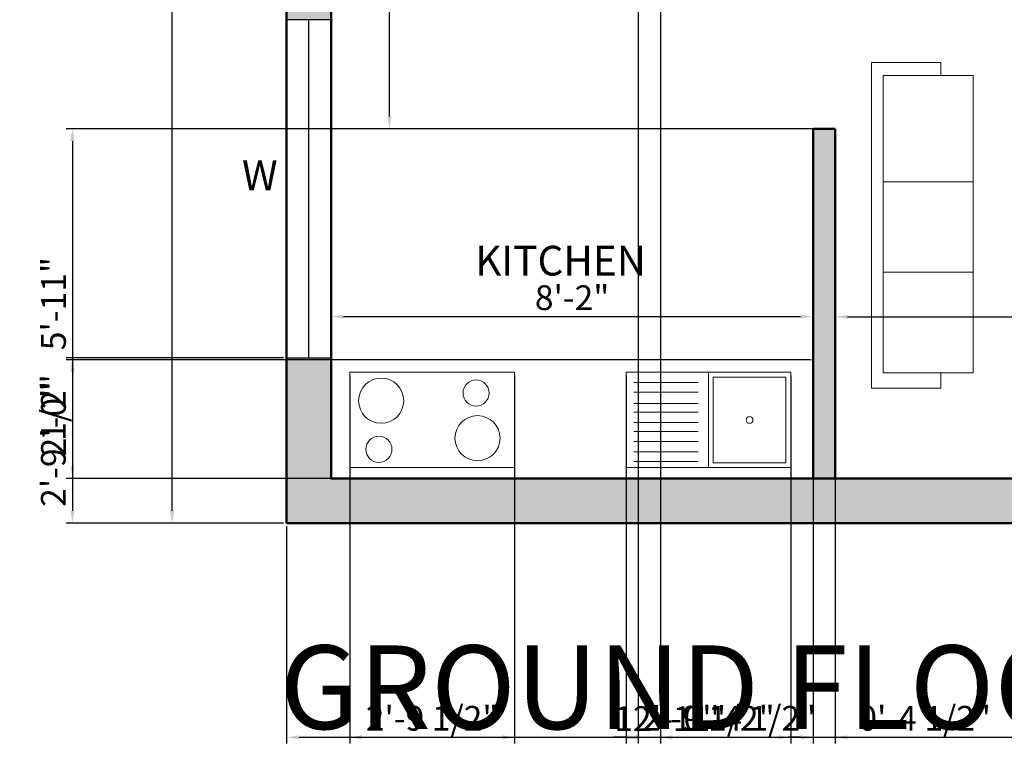
# Model space of a CAD drawing. Units: inches. Extents: x 2064 to 2999, y 1440 to 2089.
# Tile 1 of 7: x 2064 to 2263, y 1440 to 1590. Entities that reach past the tile are written whole.
import ezdxf

# ---------------------------------------------------------------- set-up
doc = ezdxf.new("R2010")
doc.units = ezdxf.units.IN
for name, color, linetype, lineweight in [('A-ANNO-DIMS', 2, 'Continuous', 18), ('A-ANNO-TEXT', 3, 'Continuous', 18), ('A-AREA-IDEN', 7, 'Continuous', 18), ('A-FLOR-FIXT', 9, 'Continuous', 18), ('A-FURN', 8, 'Continuous', 18), ('A-GLAZ', 3, 'Continuous', 25), ('A-WALL', 7, 'Continuous', 50), ('A-WALL-PATT', 8, 'Continuous', 13)]:
    doc.layers.add(name, color=color, linetype=linetype, lineweight=lineweight)
doc.styles.get("Standard").update_dxf_attribs({"font": 'arial.ttf'})
doc.dimstyles.new('ISO-25', dxfattribs={"dimtxt": 5, "dimasz": 2.5, "dimexe": 1.25, "dimexo": 0.625, "dimtad": 1, "dimdec": 0, "dimlunit": 4, "dimtxsty": 'Standard', "dimcen": 2.5, "dimadec": 0, "dimazin": 0, "dimtfac": 1, "dimtdec": 0, "dimtmove": 0, "dimatfit": 3, "dimfxl": 1, "dimarcsym": 0})

# ---------------------------------------------------------------- blocks, each defined once
blk = doc.blocks.new('*D14')
at = {"layer": 'A-ANNO-DIMS', "color": 0, "lineweight": -2, "transparency": 16777216}
for p, q in [((2126.82, 1497.7), (2126.82, 1531.08)), ((2224.32, 1497.7), (2224.32, 1531.08)), ((2129.32, 1529.83), (2221.82, 1529.83))]:
    blk.add_line(p, q, dxfattribs=at)
at = {"layer": 'A-ANNO-DIMS', "color": 0, "transparency": 16777216}
for points in [[(2129.32, 1530.25), (2129.32, 1529.42), (2126.82, 1529.83)], [(2221.82, 1530.25), (2221.82, 1529.42), (2224.32, 1529.83)]]:
    blk.add_solid(points, dxfattribs=at)
at = {"layer": 'Defpoints', "color": 0, "transparency": 16777216}
for p in [(2224.32, 1529.83), (2126.82, 1497.07), (2224.32, 1497.07)]:
    blk.add_point(p, dxfattribs=at)
at = {"layer": 'A-ANNO-DIMS', "color": 0, "transparency": 16777216, "insert": (2175.57, 1533.01), "char_height": 5, "attachment_point": 5}
blk.add_mtext('8\'-2"', dxfattribs=at)
blk = doc.blocks.new('*D15')
at = {"layer": 'A-ANNO-DIMS', "color": 0, "lineweight": -2, "transparency": 16777216}
for p, q in [((2228.82, 1497.7), (2228.82, 1531.02)), ((2468.82, 1497.7), (2468.82, 1531.02)), ((2231.32, 1529.77), (2466.32, 1529.77))]:
    blk.add_line(p, q, dxfattribs=at)
at = {"layer": 'A-ANNO-DIMS', "color": 0, "transparency": 16777216}
for points in [[(2231.32, 1530.19), (2231.32, 1529.36), (2228.82, 1529.77)], [(2466.32, 1530.19), (2466.32, 1529.36), (2468.82, 1529.77)]]:
    blk.add_solid(points, dxfattribs=at)
at = {"layer": 'Defpoints', "color": 0, "transparency": 16777216}
for p in [(2468.82, 1529.77), (2228.82, 1497.07), (2468.82, 1497.07)]:
    blk.add_point(p, dxfattribs=at)
at = {"layer": 'A-ANNO-DIMS', "color": 0, "transparency": 16777216, "insert": (2348.82, 1532.95), "char_height": 5, "attachment_point": 5}
blk.add_mtext("20'", dxfattribs=at)
blk = doc.blocks.new('*D18')
at = {"layer": 'A-ANNO-DIMS', "color": 0, "lineweight": -2, "transparency": 16777216}
for p, q in [((2117.19, 1968.07), (2093.39, 1968.07)), ((2094.64, 1490.57), (2094.64, 1965.57)), ((2117.19, 1488.07), (2093.39, 1488.07))]:
    blk.add_line(p, q, dxfattribs=at)
at = {"layer": 'A-ANNO-DIMS', "color": 0, "transparency": 16777216}
for points in [[(2094.23, 1965.57), (2095.06, 1965.57), (2094.64, 1968.07)], [(2094.23, 1490.57), (2095.06, 1490.57), (2094.64, 1488.07)]]:
    blk.add_solid(points, dxfattribs=at)
at = {"layer": 'Defpoints', "color": 0, "transparency": 16777216}
for p in [(2094.64, 1968.07), (2117.82, 1968.07), (2117.82, 1488.07)]:
    blk.add_point(p, dxfattribs=at)
at = {"layer": 'A-ANNO-DIMS', "color": 0, "transparency": 16777216, "insert": (2091.47, 1728.07), "char_height": 5, "attachment_point": 5, "rotation": 90}
blk.add_mtext("40'", dxfattribs=at)
blk = doc.blocks.new('*D39')
at = {"layer": 'A-ANNO-DIMS', "color": 0, "lineweight": -2, "transparency": 16777216}
for p, q in [((2223.69, 1702.57), (2137.36, 1702.57)), ((2138.61, 1570.34), (2138.61, 1700.07)), ((2223.69, 1567.84), (2137.36, 1567.84))]:
    blk.add_line(p, q, dxfattribs=at)
at = {"layer": 'A-ANNO-DIMS', "color": 0, "transparency": 16777216}
for points in [[(2138.19, 1700.07), (2139.03, 1700.07), (2138.61, 1702.57)], [(2138.19, 1570.34), (2139.03, 1570.34), (2138.61, 1567.84)]]:
    blk.add_solid(points, dxfattribs=at)
at = {"layer": 'Defpoints', "color": 0, "transparency": 16777216}
for p in [(2138.61, 1702.57), (2224.32, 1702.57), (2224.32, 1567.84)]:
    blk.add_point(p, dxfattribs=at)
at = {"layer": 'A-ANNO-DIMS', "color": 0, "transparency": 16777216, "insert": (2135.43, 1635.2), "char_height": 5, "attachment_point": 5, "rotation": 90}
blk.add_mtext('11\'-3"', dxfattribs=at)
blk = doc.blocks.new('SOFA-3')
for p, q in [((0, 0), (0, 65.92)), ((0, 65.92), (14.01, 65.92)), ((14.01, 65.92), (14.01, 63.25)), ((20.61, 41.74), (2.39, 41.74)), ((20.61, 23.49), (2.39, 23.49)), ((14.01, 3.1), (14.01, 0)), ((14.01, 0), (0, 0))]:
    blk.add_line(p, q)
blk.add_lwpolyline([(2.39, 3.1), (20.61, 3.1), (20.61, 63.25), (2.39, 63.25)], close=True)
blk = doc.blocks.new('WIN-68')
blk.add_line((4.5, 0), (4.5, 68.43))
blk.add_lwpolyline([(0, 0), (9, 0), (9, 68.43), (0, 68.43)], close=True)
blk = doc.blocks.new('*D77')
at = {"layer": 'A-ANNO-DIMS', "color": 0, "lineweight": -2, "transparency": 16777216}
for p, q in [((2117.19, 1521.46), (2073.22, 1521.46)), ((2074.47, 1518.96), (2074.47, 1490.57)), ((2117.19, 1488.07), (2073.22, 1488.07))]:
    blk.add_line(p, q, dxfattribs=at)
at = {"layer": 'A-ANNO-DIMS', "color": 0, "transparency": 16777216}
for points in [[(2074.05, 1518.96), (2074.89, 1518.96), (2074.47, 1521.46)], [(2074.05, 1490.57), (2074.89, 1490.57), (2074.47, 1488.07)]]:
    blk.add_solid(points, dxfattribs=at)
at = {"layer": 'Defpoints', "color": 0, "transparency": 16777216}
for p in [(2117.82, 1521.46), (2074.47, 1488.07), (2117.82, 1488.07)]:
    blk.add_point(p, dxfattribs=at)
at = {"layer": 'A-ANNO-DIMS', "color": 0, "transparency": 16777216, "insert": (2071.26, 1504.76), "char_height": 5, "attachment_point": 5, "rotation": 90}
blk.add_mtext('2\'-9 1/2"', dxfattribs=at)
blk = doc.blocks.new('*D78')
at = {"layer": 'A-ANNO-DIMS', "color": 0, "lineweight": -2, "transparency": 16777216}
for p, q in [((2117.82, 1487.45), (2117.82, 1443.47)), ((2273.05, 1487.45), (2273.05, 1443.47)), ((2120.32, 1444.72), (2270.55, 1444.72))]:
    blk.add_line(p, q, dxfattribs=at)
at = {"layer": 'A-ANNO-DIMS', "color": 0, "transparency": 16777216}
for points in [[(2120.32, 1445.14), (2120.32, 1444.3), (2117.82, 1444.72)], [(2270.55, 1445.14), (2270.55, 1444.3), (2273.05, 1444.72)]]:
    blk.add_solid(points, dxfattribs=at)
at = {"layer": 'Defpoints', "color": 0, "transparency": 16777216}
for p in [(2117.82, 1488.07), (2273.05, 1488.07), (2273.05, 1444.72)]:
    blk.add_point(p, dxfattribs=at)
at = {"layer": 'A-ANNO-DIMS', "color": 0, "transparency": 16777216, "insert": (2195.43, 1447.86), "char_height": 5, "attachment_point": 5}
blk.add_mtext('12\'-11"', dxfattribs=at)
blk = doc.blocks.new('*D96')
at = {"layer": 'A-ANNO-DIMS', "color": 0, "lineweight": -2, "transparency": 16777216}
for p, q in [((2188.93, 1709.59), (2188.93, 1443.47)), ((2193.43, 1709.59), (2193.43, 1443.47)), ((2186.43, 1444.72), (2183.93, 1444.72)), ((2188.93, 1444.72), (2193.43, 1444.72)), ((2195.93, 1444.72), (2224.63, 1444.72))]:
    blk.add_line(p, q, dxfattribs=at)
at = {"layer": 'A-ANNO-DIMS', "color": 0, "transparency": 16777216}
for points in [[(2186.43, 1445.14), (2186.43, 1444.3), (2188.93, 1444.72)], [(2195.93, 1445.14), (2195.93, 1444.3), (2193.43, 1444.72)]]:
    blk.add_solid(points, dxfattribs=at)
at = {"layer": 'Defpoints', "color": 0, "transparency": 16777216}
for p in [(2188.93, 1710.22), (2193.43, 1710.22), (2193.43, 1444.72)]:
    blk.add_point(p, dxfattribs=at)
at = {"layer": 'A-ANNO-DIMS', "color": 0, "transparency": 16777216, "insert": (2211.53, 1447.93), "char_height": 5, "attachment_point": 5}
blk.add_mtext('0\'-4 1/2"', dxfattribs=at)
blk = doc.blocks.new('*D97')
at = {"layer": 'A-ANNO-DIMS', "color": 0, "lineweight": -2, "transparency": 16777216}
for p, q in [((2224.32, 1567.21), (2224.32, 1443.47)), ((2228.82, 1567.21), (2228.82, 1443.47)), ((2221.82, 1444.72), (2219.32, 1444.72)), ((2224.32, 1444.72), (2228.82, 1444.72)), ((2231.32, 1444.72), (2260.01, 1444.72))]:
    blk.add_line(p, q, dxfattribs=at)
at = {"layer": 'A-ANNO-DIMS', "color": 0, "transparency": 16777216}
for points in [[(2221.82, 1445.14), (2221.82, 1444.3), (2224.32, 1444.72)], [(2231.32, 1445.14), (2231.32, 1444.3), (2228.82, 1444.72)]]:
    blk.add_solid(points, dxfattribs=at)
at = {"layer": 'Defpoints', "color": 0, "transparency": 16777216}
for p in [(2224.32, 1567.84), (2228.82, 1567.84), (2228.82, 1444.72)]:
    blk.add_point(p, dxfattribs=at)
at = {"layer": 'A-ANNO-DIMS', "color": 0, "transparency": 16777216, "insert": (2246.91, 1447.93), "char_height": 5, "attachment_point": 5}
blk.add_mtext('0\'-4 1/2"', dxfattribs=at)
blk = doc.blocks.new('*D99')
at = {"layer": 'A-ANNO-DIMS', "color": 0, "lineweight": -2, "transparency": 16777216}
for p, q in [((2223.69, 1521.07), (2073.22, 1521.07)), ((2074.47, 1518.57), (2074.47, 1499.57)), ((2223.69, 1497.07), (2073.22, 1497.07))]:
    blk.add_line(p, q, dxfattribs=at)
at = {"layer": 'A-ANNO-DIMS', "color": 0, "transparency": 16777216}
for points in [[(2074.05, 1518.57), (2074.89, 1518.57), (2074.47, 1521.07)], [(2074.05, 1499.57), (2074.89, 1499.57), (2074.47, 1497.07)]]:
    blk.add_solid(points, dxfattribs=at)
at = {"layer": 'Defpoints', "color": 0, "transparency": 16777216}
for p in [(2224.32, 1521.07), (2074.47, 1497.07), (2224.32, 1497.07)]:
    blk.add_point(p, dxfattribs=at)
at = {"layer": 'A-ANNO-DIMS', "color": 0, "transparency": 16777216, "insert": (2071.29, 1509.07), "char_height": 5, "attachment_point": 5, "rotation": 90}
blk.add_mtext('2\'-0"', dxfattribs=at)
blk = doc.blocks.new('*D100')
at = {"layer": 'A-ANNO-DIMS', "color": 0, "lineweight": -2, "transparency": 16777216}
for p, q in [((2130.58, 1517.94), (2130.58, 1443.47)), ((2163.9, 1517.94), (2163.9, 1443.47)), ((2133.08, 1444.72), (2161.4, 1444.72))]:
    blk.add_line(p, q, dxfattribs=at)
at = {"layer": 'A-ANNO-DIMS', "color": 0, "transparency": 16777216}
for points in [[(2133.08, 1445.14), (2133.08, 1444.3), (2130.58, 1444.72)], [(2161.4, 1445.14), (2161.4, 1444.3), (2163.9, 1444.72)]]:
    blk.add_solid(points, dxfattribs=at)
at = {"layer": 'Defpoints', "color": 0, "transparency": 16777216}
for p in [(2130.58, 1518.57), (2163.9, 1518.57), (2163.9, 1444.72)]:
    blk.add_point(p, dxfattribs=at)
at = {"layer": 'A-ANNO-DIMS', "color": 0, "transparency": 16777216, "insert": (2147.24, 1447.93), "char_height": 5, "attachment_point": 5}
blk.add_mtext('2\'-9 1/2"', dxfattribs=at)
blk = doc.blocks.new('*D101')
at = {"layer": 'A-ANNO-DIMS', "color": 0, "lineweight": -2, "transparency": 16777216}
for p, q in [((2186.48, 1517.94), (2186.48, 1443.47)), ((2219.8, 1517.94), (2219.8, 1443.47)), ((2188.98, 1444.72), (2217.3, 1444.72))]:
    blk.add_line(p, q, dxfattribs=at)
at = {"layer": 'A-ANNO-DIMS', "color": 0, "transparency": 16777216}
for points in [[(2188.98, 1445.14), (2188.98, 1444.3), (2186.48, 1444.72)], [(2217.3, 1445.14), (2217.3, 1444.3), (2219.8, 1444.72)]]:
    blk.add_solid(points, dxfattribs=at)
at = {"layer": 'Defpoints', "color": 0, "transparency": 16777216}
for p in [(2186.48, 1518.57), (2219.8, 1518.57), (2219.8, 1444.72)]:
    blk.add_point(p, dxfattribs=at)
at = {"layer": 'A-ANNO-DIMS', "color": 0, "transparency": 16777216, "insert": (2203.14, 1447.93), "char_height": 5, "attachment_point": 5}
blk.add_mtext('2\'-9 1/2"', dxfattribs=at)
blk = doc.blocks.new('*D102')
at = {"layer": 'A-ANNO-DIMS', "color": 0, "lineweight": -2, "transparency": 16777216}
for p, q in [((2228.19, 1567.84), (2073.22, 1567.84)), ((2074.47, 1565.34), (2074.47, 1499.57)), ((2228.19, 1497.07), (2073.22, 1497.07))]:
    blk.add_line(p, q, dxfattribs=at)
at = {"layer": 'A-ANNO-DIMS', "color": 0, "transparency": 16777216}
for points in [[(2074.05, 1565.34), (2074.89, 1565.34), (2074.47, 1567.84)], [(2074.05, 1499.57), (2074.89, 1499.57), (2074.47, 1497.07)]]:
    blk.add_solid(points, dxfattribs=at)
at = {"layer": 'Defpoints', "color": 0, "transparency": 16777216}
for p in [(2228.82, 1567.84), (2074.47, 1497.07), (2228.82, 1497.07)]:
    blk.add_point(p, dxfattribs=at)
at = {"layer": 'A-ANNO-DIMS', "color": 0, "transparency": 16777216, "insert": (2071.29, 1532.45), "char_height": 5, "attachment_point": 5, "rotation": 90}
blk.add_mtext('5\'-11"', dxfattribs=at)

msp = doc.modelspace()

# ---------------------------------------------------------------- hatches: boundary and pattern name
at = {"layer": 'A-WALL-PATT'}
h = msp.add_hatch(color=256, dxfattribs=at)
h.dxf.hatch_style = 1
h.paths.add_polyline_path([(2267.27, 1968.07), (2215.88, 1968.07), (2215.88, 1959.07), (2246.82, 1959.07), (2267.27, 1959.07)])
h.paths.add_polyline_path([(2477.82, 1968.07), (2300.73, 1968.07), (2300.73, 1959.07), (2317.32, 1959.07), (2468.82, 1959.07), (2468.82, 1925.2), (2477.82, 1925.2)])
h.paths.add_polyline_path([(2154.1, 1968.07), (2117.82, 1968.07), (2117.82, 1784.53), (2126.82, 1784.53), (2126.82, 1959.07), (2154.1, 1959.07)])
h.paths.add_polyline_path([(2126.82, 1716.1), (2117.82, 1716.1), (2117.82, 1685.76), (2126.82, 1685.76)])
h.paths.add_polyline_path([(2126.82, 1617.33), (2117.82, 1617.33), (2117.82, 1589.89), (2126.82, 1589.89)])
h.paths.add_polyline_path([(2273.05, 1497.07), (2228.82, 1497.07), (2126.82, 1497.07), (2126.82, 1521.07), (2126.82, 1521.46), (2117.82, 1521.46), (2117.82, 1488.07), (2273.05, 1488.07)])
h.paths.add_polyline_path([(2409.19, 1494.07, -0.01877), (2409.3, 1497.07), (2356.92, 1497.07), (2356.92, 1488.07), (2409.19, 1488.07)])
h.paths.add_polyline_path([(2468.82, 1638.07), (2348.82, 1638.07), (2348.82, 1668.53), (2348.82, 1710.05), (2344.32, 1710.05), (2344.32, 1633.57), (2468.82, 1633.57)])
h.paths.add_polyline_path([(2228.82, 1567.84), (2224.32, 1567.84), (2224.32, 1497.07), (2228.82, 1497.07)])
h.paths.add_polyline_path([(2477.82, 1781.8), (2468.82, 1781.8), (2468.82, 1762.57), (2468.82, 1728.07), (2477.82, 1728.07)])
h.paths.add_polyline_path([(2468.82, 1762.57), (2372.82, 1762.57), (2372.82, 1801.78), (2368.32, 1801.78), (2368.32, 1758.07), (2468.82, 1758.07)])
h.paths.add_polyline_path([(2477.82, 1865.66), (2468.82, 1865.66), (2468.82, 1814.01), (2477.82, 1814.01)])
h.paths.add_polyline_path([(2321.82, 1959.07), (2317.32, 1959.07), (2317.32, 1839.07), (2251.32, 1839.07), (2251.32, 1834.57), (2321.82, 1834.57)])
h.paths.add_polyline_path([(2200.07, 1839.07), (2126.82, 1839.07), (2126.82, 1834.57), (2200.07, 1834.57)])
h.paths.add_polyline_path([(2193.43, 1834.57), (2188.93, 1834.57), (2188.93, 1710.22), (2193.43, 1710.22)])
h.paths.add_polyline_path([(2251.32, 1959.07), (2246.82, 1959.07), (2246.82, 1950.75), (2251.21, 1950.75), (2251.32, 1950.75)])
h.paths.add_polyline_path([(2251.32, 1921.46), (2246.82, 1921.46), (2246.82, 1839.07), (2240.07, 1839.07), (2240.07, 1834.57), (2251.32, 1834.57), (2251.32, 1839.07)])
h.paths.add_polyline_path([(2468.82, 1839.07), (2363.36, 1839.07), (2363.36, 1834.57), (2468.82, 1834.57)])
h.paths.add_polyline_path([(2323.36, 1839.07), (2321.82, 1839.07), (2321.82, 1834.57), (2323.36, 1834.57)])
h = msp.add_hatch(color=256, dxfattribs=at)
h.dxf.hatch_style = 1
h.paths.add_polyline_path([(2449.19, 1497.07), (2449.19, 1494.07), (2449.19, 1488.07), (2468.82, 1488.07), (2468.82, 1497.07)])
h.paths.add_polyline_path([(2468.82, 1488.07), (2477.82, 1488.07), (2477.82, 1668.53), (2468.82, 1668.53)])
h.paths.add_polyline_path([(2454.62, 1692.05), (2454.62, 1703.66), (2444.32, 1703.66), (2444.32, 1692.05)], flags=9)
h.paths.add_polyline_path([(2167.39, 1527.81), (2183.8, 1527.81), (2183.8, 1538.12), (2167.39, 1538.12)], flags=9)
h.paths.add_polyline_path([(2343.08, 1527.75), (2354.68, 1527.75), (2354.68, 1538.06), (2343.08, 1538.06)], flags=9)
h.paths.add_polyline_path([(2462.54, 1554.96), (2462.54, 1575.25), (2452.24, 1575.25), (2452.24, 1554.96)], flags=9)
h.paths.add_polyline_path([(2140.63, 1624.84), (2140.63, 1645.13), (2130.32, 1645.13), (2130.32, 1624.84)], flags=9)
h.paths.add_polyline_path([(2137.9, 1938.01), (2190.4, 1938.01), (2190.4, 1950.4), (2137.9, 1950.4)], flags=9)
h.paths.add_polyline_path([(2337.44, 1898.9), (2337.44, 1951.39), (2325.04, 1951.39), (2325.04, 1898.9)], flags=9)
h.paths.add_polyline_path([(2380.15, 1768.58), (2405.57, 1768.58), (2405.57, 1780.97), (2380.15, 1780.97)], flags=9)
h.paths.add_polyline_path([(2370.32, 1679.42), (2432.16, 1679.42), (2432.16, 1691.82), (2370.32, 1691.82)], flags=9)
h.paths.add_polyline_path([(2322.2, 1541.98), (2382.63, 1541.98), (2382.63, 1554.37), (2322.2, 1554.37)], flags=9)
h.paths.add_polyline_path([(2153.83, 1534.75), (2193.72, 1534.75), (2193.72, 1547.14), (2153.83, 1547.14)], flags=9)
h.paths.add_polyline_path([(2162.47, 1614.19), (2217.78, 1614.19), (2217.78, 1626.58), (2162.47, 1626.58)], flags=9)
h.paths.add_polyline_path([(2217.9, 1723.52), (2261.07, 1723.52), (2261.07, 1735.92), (2217.9, 1735.92)], flags=9)
h.paths.add_polyline_path([(2270.61, 1869.16), (2296.03, 1869.16), (2296.03, 1881.55), (2270.61, 1881.55)], flags=9)
h.paths.add_polyline_path([(2353.7, 1922), (2422.07, 1922), (2422.07, 1934.4), (2353.7, 1934.4)], flags=9)
h.paths.add_polyline_path([(2133.7, 1917.44), (2217.48, 1917.44), (2217.48, 1929.83), (2133.7, 1929.83)], flags=9)

# ---------------------------------------------------------------- linework, layer by layer
at = {"layer": 'A-FLOR-FIXT'}
for p, q in [((2126.82, 1521.07), (2224.32, 1521.07)), ((2203.14, 1499.27), (2203.14, 1518.57)), ((2188.08, 1516.51), (2201.05, 1516.51)), ((2188.08, 1514.55), (2201.05, 1514.55)), ((2188.08, 1512.28), (2201.05, 1512.28)), ((2188.08, 1510.47), (2201.05, 1510.47)), ((2188.08, 1508.43), (2201.05, 1508.43)), ((2188.08, 1506.57), (2201.05, 1506.57)), ((2188.08, 1504.59), (2201.05, 1504.59)), ((2188.08, 1502.49), (2201.05, 1502.49)), ((2188.08, 1500.51), (2201.05, 1500.51))]:
    msp.add_line(p, q, dxfattribs=at)
for points in [[(2130.58, 1499.27), (2163.9, 1499.27), (2163.9, 1518.57), (2130.58, 1518.57)], [(2186.48, 1499.27), (2219.8, 1499.27), (2219.8, 1518.57), (2186.48, 1518.57)], [(2203.14, 1499.27), (2219.8, 1499.27), (2219.8, 1518.57), (2203.14, 1518.57)], [(2204.14, 1500.27), (2218.8, 1500.27), (2218.8, 1517.57), (2204.14, 1517.57)]]:
    msp.add_lwpolyline(points, close=True, dxfattribs=at)
for centre, radius in [((2136.94, 1512.81), 4.57), ((2156.15, 1514.37), 2.64), ((2156.44, 1505.24), 4.57), ((2211.47, 1508.92), 0.695), ((2136.48, 1502.98), 2.64)]:
    msp.add_circle(centre, radius, dxfattribs=at)
at = {"layer": 'A-WALL'}
for p, q in [((2117.82, 1488.07), (2117.82, 1968.07)), ((2224.32, 1497.07), (2224.32, 1567.84)), ((2224.32, 1567.84), (2228.82, 1567.84)), ((2228.82, 1497.07), (2228.82, 1567.84)), ((2126.82, 1497.07), (2126.82, 1521.07)), ((2409.3, 1497.07), (2228.82, 1497.07)), ((2409.19, 1488.07), (2117.82, 1488.07))]:
    msp.add_line(p, q, dxfattribs=at)
for points in [[(2449.19, 1488.07), (2477.82, 1488.07), (2477.82, 1968.07), (2117.82, 1968.07), (2117.82, 1488.07), (2409.19, 1488.07)], [(2447.44, 1497.07), (2468.82, 1497.07), (2468.82, 1959.07), (2126.82, 1959.07), (2126.82, 1497.07), (2409.3, 1497.07)]]:
    msp.add_lwpolyline(points, dxfattribs=at)

# ---------------------------------------------------------------- block references
at = {"layer": 'A-FURN'}
msp.add_blockref('SOFA-3', (2236.14, 1515.33), dxfattribs=at)
at = {"layer": 'A-GLAZ'}
msp.add_blockref('WIN-68', (2117.82, 1521.46), dxfattribs=at)

# ---------------------------------------------------------------- texts
at = {"layer": 'A-ANNO-TEXT', "attachment_point": 1}
for s, width, gutter_width, heights, insert, char_height in [('W', 152.6727, 30.08, [0], (2108.78, 1561.41), 6.02), ('GROUND FLOOR PLAN', 429.6774, 84.65, [17.52], (2116.47, 1463.31), 16.9292)]:
    msp.add_mtext_dynamic_manual_height_columns(s, width=width, gutter_width=gutter_width, heights=heights, dxfattribs=dict(at, insert=insert, char_height=char_height))
at = {"layer": 'A-AREA-IDEN', "insert": (2155.95, 1544.15), "char_height": 6.015, "attachment_point": 1}
msp.add_mtext_dynamic_manual_height_columns('KITCHEN', width=152.6727, gutter_width=30.08, heights=[0], dxfattribs=at)

# ---------------------------------------------------------------- dimensions: what is measured, and where the dimension line sits
at = {"layer": 'A-ANNO-DIMS'}
for base, p1, p2, override, picture, middle in [((2094.64, 1968.07), (2117.82, 1488.07), (2117.82, 1968.07), {"dimclrd": 0, "dimclre": 0, "dimclrt": 0}, '*D18', (2091.47, 1728.07)), ((2138.61, 1702.57), (2224.32, 1567.84), (2224.32, 1702.57), {"dimclrd": 0, "dimclre": 0, "dimclrt": 0}, '*D39', (2135.43, 1635.2)), ((2074.47, 1497.07), (2228.82, 1567.84), (2228.82, 1497.07), {"dimdec": 1, "dimlfac": 1, "dimrnd": 0, "dimzin": 1, "dimdsep": 46, "dimlunit": 4, "dimfrac": 2}, '*D102', (2071.29, 1532.45)), ((2074.47, 1488.07), (2117.82, 1521.46), (2117.82, 1488.07), {"dimdec": 1, "dimlfac": 1, "dimrnd": 0, "dimzin": 1, "dimdsep": 46, "dimlunit": 4, "dimfrac": 2}, '*D77', (2071.26, 1504.76)), ((2074.47, 1497.07), (2224.32, 1521.07), (2224.32, 1497.07), {"dimdec": 1, "dimlfac": 1, "dimrnd": 0, "dimzin": 1, "dimdsep": 46, "dimlunit": 4, "dimfrac": 2}, '*D99', (2071.29, 1509.07))]:
    dim = msp.add_linear_dim(base=base, p1=p1, p2=p2, angle=90, dimstyle='ISO-25', override=override, dxfattribs=at)
    dim.commit()
    dim.dimension.update_dxf_attribs({"geometry": picture, "text_midpoint": middle})
for base, p1, p2, override, picture, middle in [((2193.43, 1444.72), (2188.93, 1710.22), (2193.43, 1710.22), {"dimdec": 1, "dimlfac": 1, "dimrnd": 0, "dimzin": 1, "dimdsep": 46, "dimlunit": 4, "dimfrac": 2}, '*D96', (2211.53, 1447.93)), ((2228.82, 1444.72), (2224.32, 1567.84), (2228.82, 1567.84), {"dimdec": 1, "dimlfac": 1, "dimrnd": 0, "dimzin": 1, "dimdsep": 46, "dimlunit": 4, "dimfrac": 2}, '*D97', (2246.91, 1447.93)), ((2224.31868146, 1529.83204802), (2126.81868146, 1497.070928), (2224.31868146, 1497.070928), {"dimclrd": 0, "dimclre": 0, "dimclrt": 0}, '*D14', (2175.56868146, 1533.00991296)), ((2468.82, 1529.77), (2228.82, 1497.07), (2468.82, 1497.07), {"dimclrd": 0, "dimclre": 0, "dimclrt": 0}, '*D15', (2348.82, 1532.95)), ((2163.9, 1444.72), (2130.58, 1518.57), (2163.9, 1518.57), {"dimdec": 1, "dimlfac": 1, "dimrnd": 0, "dimzin": 1, "dimdsep": 46, "dimlunit": 4, "dimfrac": 2}, '*D100', (2147.24, 1447.93)), ((2219.8, 1444.72), (2186.48, 1518.57), (2219.8, 1518.57), {"dimdec": 1, "dimlfac": 1, "dimrnd": 0, "dimzin": 1, "dimdsep": 46, "dimlunit": 4, "dimfrac": 2}, '*D101', (2203.14, 1447.93)), ((2273.05, 1444.72), (2117.82, 1488.07), (2273.05, 1488.07), {"dimdec": 1, "dimlfac": 1, "dimrnd": 0, "dimzin": 1, "dimdsep": 46, "dimlunit": 4, "dimfrac": 2}, '*D78', (2195.43, 1447.86))]:
    dim = msp.add_linear_dim(base=base, p1=p1, p2=p2, dimstyle='ISO-25', override=override, dxfattribs=at)
    dim.commit()
    dim.dimension.update_dxf_attribs({"geometry": picture, "text_midpoint": middle})

doc.saveas('drawing.dxf')
